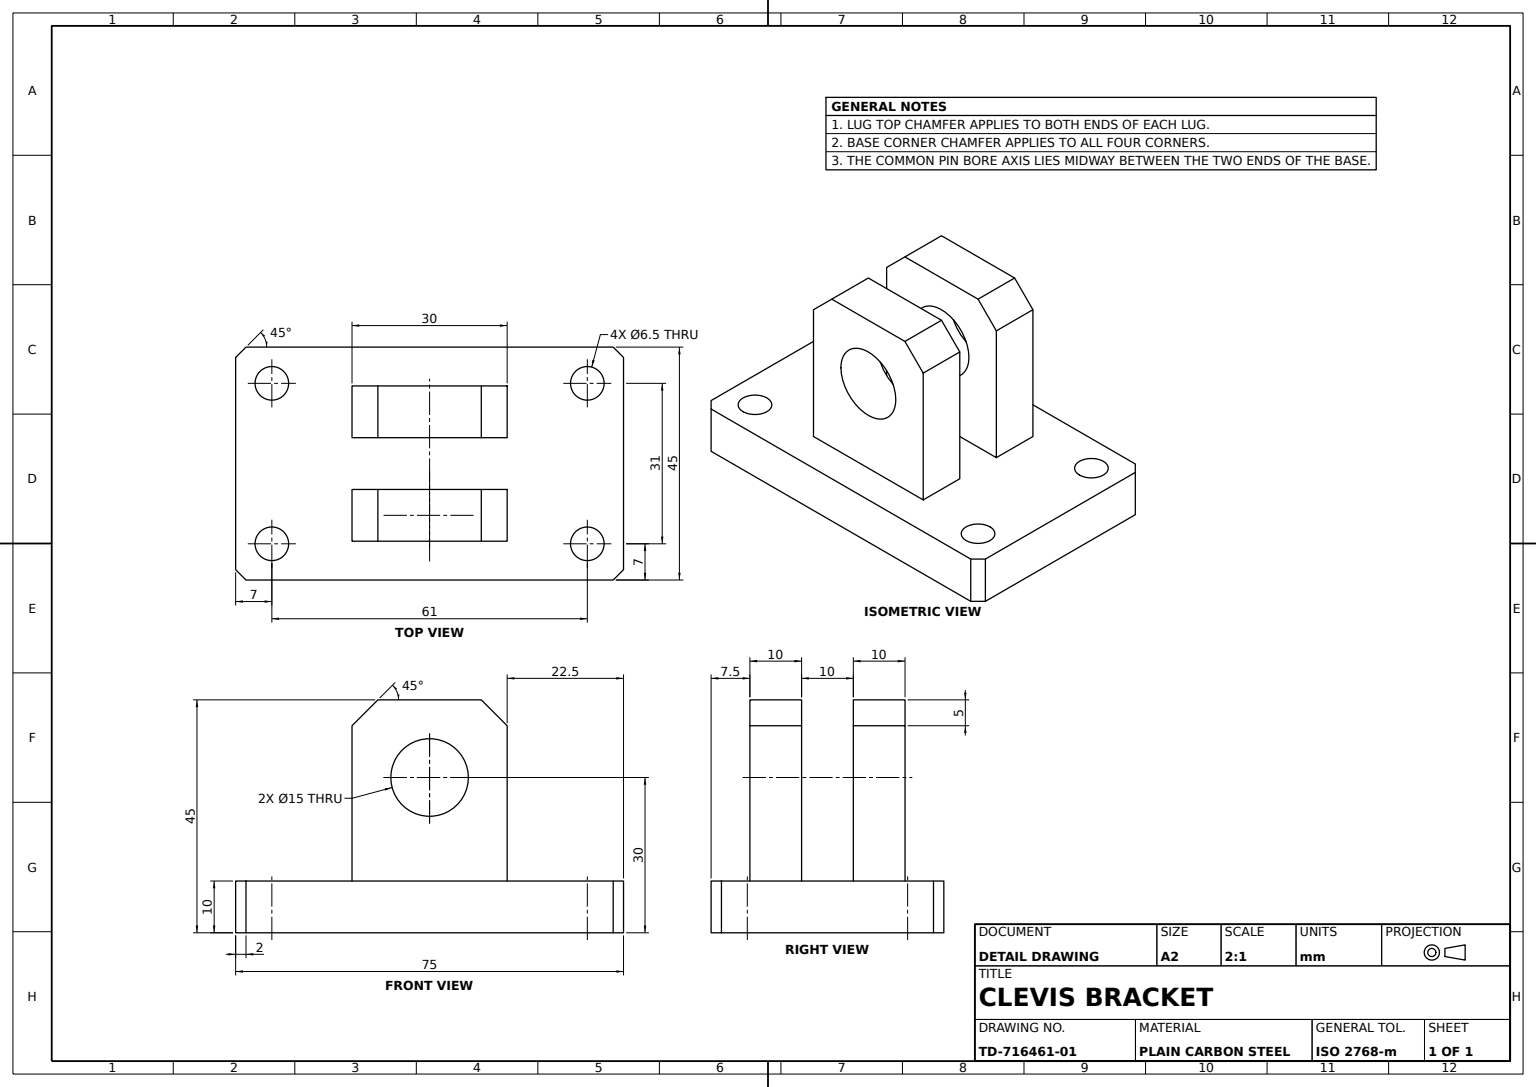
from build123d import *

# Parameters (mm, degrees)
BASE_PLATE_SKETCH_W                        = 75
BASE_PLATE_SKETCH_H                        = 45
BASE_PLATE_75X45X10_DEPTH                  = 10
LUG_PROFILE_SKETCH_W                       = 30
LUG_PROFILE_SKETCH_H                       = 10
CLEVIS_LUG_DEPTH                           = 35
LUG_TOP_CHAMFERS_5MM_SIZE                  = 5
BASE_PLATE_EDGE_CHAMFER_2MM_SIZE           = 2
MOUNTING_HOLE_SKETCH_R                     = 3.25
MOUNTING_HOLE_6_5_DEPTH                    = 57.013391256
MOUNTING_HOLES_MIRROR_RIGHT_COPY_1_SKETC_R = 3.25
MOUNTING_HOLES_MIRROR_RIGHT_COPY_1_DEPTH   = 57.013391256
PIN_BORE_SKETCH_R                          = 7.5
PIN_BORE_15_DEPTH                          = 70.552138716


with BuildPart() as part:
    # Base Plate Sketch → Base Plate 75x45x10 (new body)
    with BuildSketch(Plane(origin=(0, 0, 0), x_dir=(1, 0, 0), z_dir=(0, 1, 0))):
        Rectangle(BASE_PLATE_SKETCH_W, BASE_PLATE_SKETCH_H)
    extrude(amount=BASE_PLATE_75X45X10_DEPTH)

    # Lug Profile Sketch → Clevis Lug (add)
    with BuildSketch(Plane(origin=(0, 10, 0), x_dir=(1, 0, 0), z_dir=(0, 1, 0))):
        with Locations((0, -10)):
            Rectangle(LUG_PROFILE_SKETCH_W, LUG_PROFILE_SKETCH_H)
    clevis_lug = extrude(amount=CLEVIS_LUG_DEPTH)

    # Clevis Lug Mirror: Clevis Lug across plane
    add(clevis_lug.mirror(Plane.XY))

    # Lug Top Chamfers 5mm
    lug_top_chamfers_5mm_edges = [part.edges().sort_by_distance(p)[0] for p in [
        (15, 45, 10),
        (-15, 45, 10),
        (15, 45, -10),
        (-15, 45, -10),
    ]]
    chamfer(lug_top_chamfers_5mm_edges, length=LUG_TOP_CHAMFERS_5MM_SIZE)

    # Base Plate Edge Chamfer 2mm
    base_plate_edge_chamfer_2mm_edges = [part.edges().sort_by_distance(p)[0] for p in [
        (-37.5, 5, -22.5),
        (37.5, 5, -22.5),
        (37.5, 5, 22.5),
        (-37.5, 5, 22.5),
    ]]
    chamfer(base_plate_edge_chamfer_2mm_edges, length=BASE_PLATE_EDGE_CHAMFER_2MM_SIZE)

    # Mounting Hole Sketch → Mounting Hole Ø6.5 (cut, through all)
    with BuildSketch(Plane(origin=(0, 10, 0), x_dir=(1, 0, 0), z_dir=(0, 1, 0))):
        with Locations(Location((-30.5, 15.5, 0), (0, 0, 270))):
            Circle(MOUNTING_HOLE_SKETCH_R)
    mounting_hole_6_5 = extrude(amount=-MOUNTING_HOLE_6_5_DEPTH, mode=Mode.SUBTRACT)

    # Mounting Hole Mirror Front: Mounting Hole Ø6.5 across plane
    add(mounting_hole_6_5.mirror(Plane.XY), mode=Mode.SUBTRACT)

    # Mounting Holes Mirror Right: Mounting Hole Ø6.5 across plane
    add(mounting_hole_6_5.mirror(Plane(origin=(0, 0, 0), x_dir=(0, 0, 1), z_dir=(1, 0, 0))), mode=Mode.SUBTRACT)

    # Mounting Holes Mirror Right copy 1 sketc → Mounting Holes Mirror Right copy 1 (cut, through all)
    with BuildSketch(Plane(origin=(0, 10, 0), x_dir=(-1, 0, 0), z_dir=(0, 1, 0))):
        with Locations(Location((-30.5, 15.5, 0), (0, 0, 270))):
            Circle(MOUNTING_HOLES_MIRROR_RIGHT_COPY_1_SKETC_R)
    extrude(amount=-MOUNTING_HOLES_MIRROR_RIGHT_COPY_1_DEPTH, mode=Mode.SUBTRACT)

    # Pin Bore Sketch → Pin Bore Ø15 (cut, through all)
    with BuildSketch(Plane.XY.offset(15)):
        with Locations((0, 30)):
            Circle(PIN_BORE_SKETCH_R)
    extrude(amount=-PIN_BORE_15_DEPTH, mode=Mode.SUBTRACT)


solid = part.part
